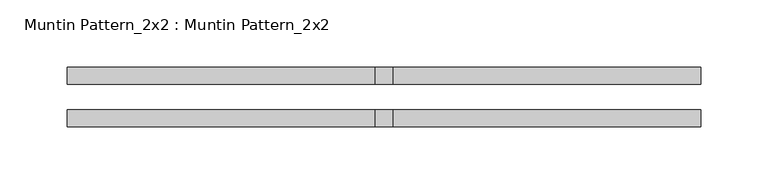
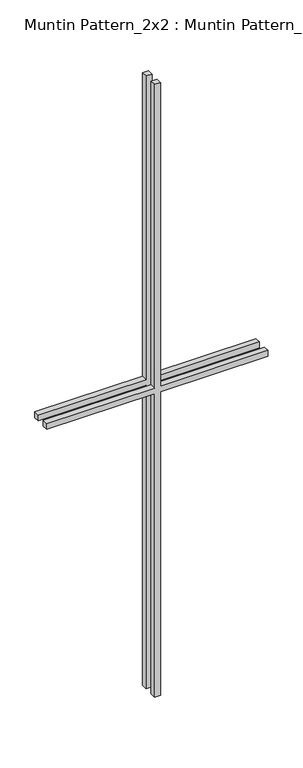
"""IFC4 building model written with IfcOpenShell, lengths in millimetres: proxy geometry, Muntin Pattern_2x2 : Muntin Pattern_2x2."""

from ifc_helpers import new_model, si_unit, frame, origin, place, context, project, spatial, polyline, outline, extrude, source, transform, mapped, element, save


def muntin_pattern_2x2_muntin_pattern_2x2_6dad3731(model_context):
    return source(origin(), model_context, "Body", "SweptSolid", [
        extrude(outline(polyline([(698.5, -6.35), (698.5, -236.5375), (685.8, -236.5375), (685.8, -6.35), (0.0, -6.35), (0.0, 6.35), (685.8, 6.35), (685.8, 236.5375), (698.5, 236.5375), (698.5, 6.35), (1384.3, 6.35), (1384.3, -6.35), (698.5, -6.35)])), frame((0.0, 9.525, 0.0), z_axis=(0.0, 1.0, 0.0), x_axis=(0.0, 0.0, 1.0)), (0.0, 0.0, 1.0), 12.7),
        extrude(outline(polyline([(698.5, -6.35), (698.5, -236.5375), (685.8, -236.5375), (685.8, -6.35), (0.0, -6.35), (0.0, 6.35), (685.8, 6.35), (685.8, 236.5375), (698.5, 236.5375), (698.5, 6.35), (1384.3, 6.35), (1384.3, -6.35), (698.5, -6.35)])), frame((0.0, -22.225, 0.0), z_axis=(0.0, 1.0, 0.0), x_axis=(0.0, 0.0, 1.0)), (0.0, 0.0, 1.0), 12.7),
    ])


if __name__ == "__main__":
    model = new_model("IFC4")
    model_context = context("Model", 3, world=origin())
    ifc_project = project(units=[si_unit("LENGTHUNIT", "METRE", prefix="MILLI")], contexts=[model_context])
    site = spatial("IfcSite", under=ifc_project)
    building = spatial("IfcBuilding", under=site)
    placement = place(None, origin())
    muntin_pattern_2x2_muntin_pattern_2x2_shape = muntin_pattern_2x2_muntin_pattern_2x2_6dad3731(model_context)
    element("IfcBuildingElementProxy", 1, Name="Muntin Pattern_2x2 : Muntin Pattern_2x2", ObjectType="Muntin Pattern_2x2 : Muntin Pattern_2x2", at=placement, inside=building, context=model_context, shape_type="MappedRepresentation", body=[
        mapped(muntin_pattern_2x2_muntin_pattern_2x2_shape, transform((0.0, 0.0, 0.0), x_axis=(1.0, 0.0, 0.0), y_axis=(0.0, 1.0, 0.0), z_axis=(0.0, 0.0, 1.0))),
    ])
    save(model, "model.ifc")

# Revit data of these elements
# Type "Muntin Pattern_2x2 : Muntin Pattern_2x2"
#   Width [instance default] = 4' - 0"
#   Thickness = 0' - 0 1/2"
#   Height [instance default] = 4' - 0"
#   Distance = 0' - 0 3/4"
#   Interior Material [instance default] = none
#   Exterior Material [instance default] = none
#   Default Elevation = 0
# Element 1 (IfcBuildingElementProxy, "Muntin Pattern_2x2 : Muntin Pattern_2x2")
#   Width = 1' - 6 5/8"
#   Height = 4' - 6 1/2"
#   Interior Material = Wood - Stained
#   Exterior Material = Clad - White
#   Materials on its faces: "Clad - White", "Wood - Stained"
# Materials
#   "Clad - White": class "Wood", colour RGB 242 242 238, transparency 0, Cost = 0
#   "Wood - Stained": class "Wood", colour RGB 224 178 126, transparency 0, Cost = 0
